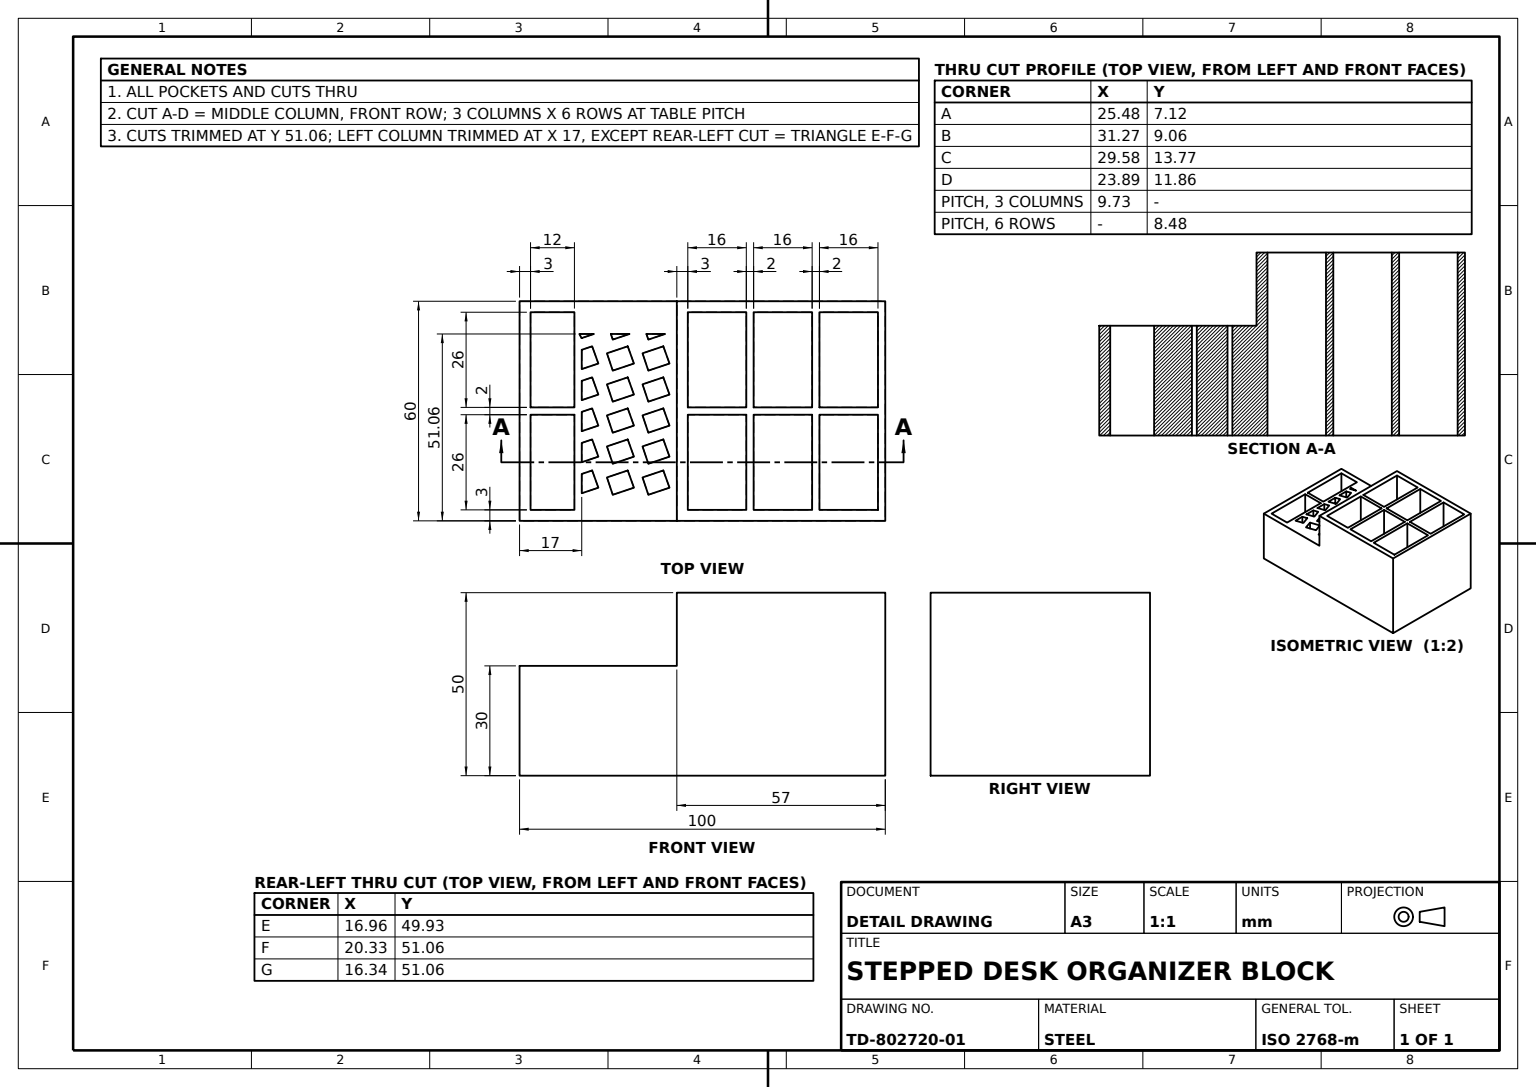
from build123d import *

# Parameters (mm, degrees)
STEPPED_BLOCK_DEPTH         = 30
LOWER_STEP_POCKETS_SKETCH_W = 16
LOWER_STEP_POCKETS_SKETCH_H = 26
LOWER_STEP_POCKETS_DEPTH    = 77.811457479
UPPER_STEP_POCKETS_SKETCH_W = 12
UPPER_STEP_POCKETS_SKETCH_H = 26
UPPER_STEP_POCKETS_DEPTH    = 66.574385243
TRIANGULAR_CUTS_DEPTH       = 30


with BuildPart() as part:
    # Stepped Block Profile → Stepped Block (new, symmetric)
    with BuildSketch(Plane.XY):
        Polygon((-50, 5.599472991), (50, 5.599472991), (50, 55.599472991), (-7, 55.599472991), (-7, 35.599472991), (-50, 35.599472991), align=None)
    extrude(amount=STEPPED_BLOCK_DEPTH, both=True)

    # Lower Step Pockets Sketch → Lower Step Pockets (cut, through all)
    with BuildSketch(Plane(origin=(0, 55.599472991, 0), x_dir=(1, 0, 0), z_dir=(0, 1, 0))):
        with Locations((4, -14)):
            Rectangle(LOWER_STEP_POCKETS_SKETCH_W, LOWER_STEP_POCKETS_SKETCH_H)
        with Locations((22, -14)):
            Rectangle(LOWER_STEP_POCKETS_SKETCH_W, LOWER_STEP_POCKETS_SKETCH_H)
        with Locations((40, -14)):
            Rectangle(LOWER_STEP_POCKETS_SKETCH_W, LOWER_STEP_POCKETS_SKETCH_H)
        with Locations((40, 14)):
            Rectangle(LOWER_STEP_POCKETS_SKETCH_W, LOWER_STEP_POCKETS_SKETCH_H)
        with Locations((22, 14)):
            Rectangle(LOWER_STEP_POCKETS_SKETCH_W, LOWER_STEP_POCKETS_SKETCH_H)
        with Locations((4, 14)):
            Rectangle(LOWER_STEP_POCKETS_SKETCH_W, LOWER_STEP_POCKETS_SKETCH_H)
    extrude(amount=-LOWER_STEP_POCKETS_DEPTH, mode=Mode.SUBTRACT)

    # Upper Step Pockets Sketch → Upper Step Pockets (cut, through all)
    with BuildSketch(Plane(origin=(0, 35.599472991, 0), x_dir=(1, 0, 0), z_dir=(0, 1, 0))):
        with Locations((-41, -14)):
            Rectangle(UPPER_STEP_POCKETS_SKETCH_W, UPPER_STEP_POCKETS_SKETCH_H)
        with Locations((-41, 14)):
            Rectangle(UPPER_STEP_POCKETS_SKETCH_W, UPPER_STEP_POCKETS_SKETCH_H)
    extrude(amount=-UPPER_STEP_POCKETS_DEPTH, mode=Mode.SUBTRACT)

    # Triangular Cuts Sketch → Triangular Cuts (cut)
    with BuildSketch(Plane(origin=(0, 35.599472991, 0), x_dir=(1, 0, 0), z_dir=(0, 1, 0))):
        Polygon((-33.663373821, 21.060066869), (-29.666961616, 21.060066869), (-33.0416794, 19.929357963), align=None)
        Polygon((-33, 16.73436244), (-33, 11.462429856), (-28.457896441, 12.984274726), (-30.149434639, 17.689452568), align=None)
        Polygon((-18.728948221, -20.939296913), (-24.521548709, -22.880124378), (-26.109644568, -18.140287882), (-20.420486418, -16.234119071), align=None)
        Polygon((-9, -20.939296913), (-14.792600489, -22.880124378), (-16.380696348, -18.140287882), (-10.691538197, -16.234119071), align=None)
        Polygon((-28.457896441, -20.939296913), (-33, -22.461141782), (-33, -17.189209199), (-30.149434639, -16.234119071), align=None)
        Polygon((-18.728948221, -12.458404003), (-24.521548709, -14.399231468), (-26.109644568, -9.659394973), (-20.420486418, -7.753226161), align=None)
        Polygon((-33, 8.25346953), (-33, 2.981536947), (-28.457896441, 4.503381816), (-30.149434639, 9.208559658), align=None)
        Polygon((-28.457896441, -12.458404003), (-33, -13.980248873), (-33, -8.708316289), (-30.149434639, -7.753226161), align=None)
        Polygon((-18.728948221, -3.977511094), (-24.521548709, -5.918338558), (-26.109644568, -1.178502063), (-20.420486418, 0.727666749), align=None)
        Polygon((-28.457896441, -3.977511094), (-33, -5.499355963), (-33, -0.22742338), (-30.149434639, 0.727666749), align=None)
        Polygon((-18.728948221, 4.503381816), (-24.521548709, 2.562554351), (-26.109644568, 7.302390847), (-20.420486418, 9.208559658), align=None)
        Polygon((-18.728948221, 12.984274726), (-24.521548709, 11.043447261), (-26.109644568, 15.783283756), (-20.420486418, 17.689452568), align=None)
        Polygon((-19.938013396, 21.060066869), (-24.521548709, 19.524340171), (-25.036098359, 21.060066869), align=None)
        Polygon((-9, -12.458404003), (-14.792600489, -14.399231468), (-16.380696348, -9.659394973), (-10.691538197, -7.753226161), align=None)
        Polygon((-9, -3.977511094), (-14.792600489, -5.918338558), (-16.380696348, -1.178502063), (-10.691538197, 0.727666749), align=None)
        Polygon((-9, 4.503381816), (-14.792600489, 2.562554351), (-16.380696348, 7.302390847), (-10.691538197, 9.208559658), align=None)
        Polygon((-9, 12.984274726), (-14.792600489, 11.043447261), (-16.380696348, 15.783283756), (-10.691538197, 17.689452568), align=None)
        Polygon((-10.209065175, 21.060066869), (-14.792600489, 19.524340171), (-15.307150139, 21.060066869), align=None)
    extrude(amount=-TRIANGULAR_CUTS_DEPTH, mode=Mode.SUBTRACT)


solid = part.part
